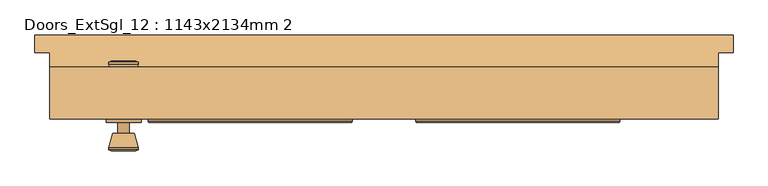
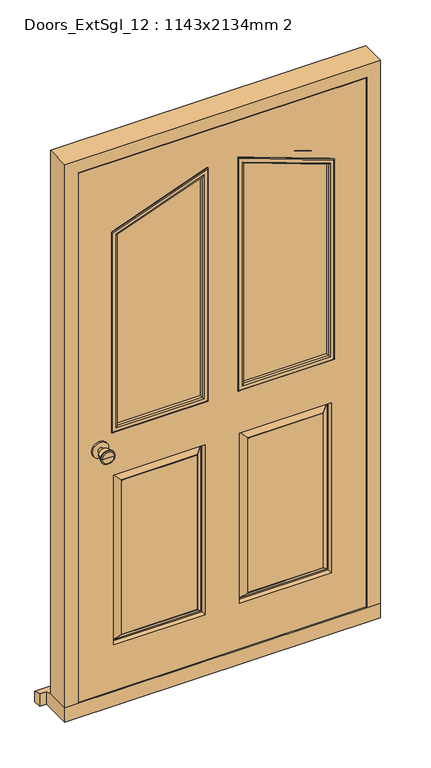
"""IFC4 building model written with IfcOpenShell, lengths in millimetres: door geometry, Doors_ExtSgl_12 : 1143x2134mm 2."""

from ifc_helpers import new_model, si_unit, point, frame, frame_2d, origin, place, context, project, spatial, polyline, circle_curve, ellipse_curve, trimmed, segment, composite_curve, outline, extrude, faceted_brep, source, transform, mapped, element, save
from ifc_brep_helpers import plane_surface, cylinder_surface, revolved_surface, advanced_brep


def doors_extsgl_12_1143x2134mm_2_6d3613a0(model_context):
    return source(origin(), model_context, "Body", "SolidModel", [
        advanced_brep(
        [(-445.0, -5.7, 1000.0), (-435.0, -5.7, 1000.0), (-455.0, -5.7, 1000.0), (-424.5241324, -54.7, 1000.0), (-445.0, -54.7, 1000.0), (-465.4758676, -54.7, 1000.0), (-420.0, -52.8721319, 1000.0), (-470.0, -52.8721319, 1000.0), (-420.0, -49.4084537, 1000.0), (-470.0, -49.4084537, 1000.0), (-426.363764, -24.7, 1000.0), (-463.636236, -24.7, 1000.0), (-435.0, -24.7, 1000.0), (-455.0, -24.7, 1000.0)],
        [
            (0, 1),
            (1, 2, circle_curve(frame((-445.0, -5.7, 1000.0), z_axis=(0.0, 1.0, 0.0), x_axis=(-1.0, 0.0, 0.0)), 10.0)),
            (2, 0),
            (2, 1, circle_curve(frame((-445.0, -5.7, 1000.0), z_axis=(0.0, 1.0, 0.0), x_axis=(-1.0, 0.0, 0.0)), 10.0)),
            (3, 4),
            (4, 5),
            (5, 3, circle_curve(frame((-445.0, -54.7, 1000.0), z_axis=(0.0, -1.0, 0.0), x_axis=(-1.0, 0.0, 0.0)), 20.4758676)),
            (3, 5, circle_curve(frame((-445.0, -54.7, 1000.0), z_axis=(0.0, -1.0, 0.0), x_axis=(-1.0, 0.0, 0.0)), 20.4758676)),
            (6, 3),
            (5, 7),
            (7, 6, circle_curve(frame((-445.0, -52.8721319, 1000.0), z_axis=(0.0, -1.0, 0.0), x_axis=(-1.0, 0.0, 0.0)), 25.0)),
            (6, 7, circle_curve(frame((-445.0, -52.8721319, 1000.0), z_axis=(0.0, -1.0, 0.0), x_axis=(-1.0, 0.0, 0.0)), 25.0)),
            (8, 6),
            (7, 9),
            (9, 8, circle_curve(frame((-445.0, -49.4084537, 1000.0), z_axis=(0.0, -1.0, 0.0), x_axis=(-1.0, 0.0, 0.0)), 25.0)),
            (8, 9, circle_curve(frame((-445.0, -49.4084537, 1000.0), z_axis=(0.0, -1.0, 0.0), x_axis=(-1.0, 0.0, 0.0)), 25.0)),
            (10, 8),
            (9, 11),
            (11, 10, circle_curve(frame((-445.0, -24.7, 1000.0), z_axis=(0.0, -1.0, 0.0), x_axis=(-1.0, 0.0, 0.0)), 18.636236)),
            (10, 11, circle_curve(frame((-445.0, -24.7, 1000.0), z_axis=(0.0, -1.0, 0.0), x_axis=(-1.0, 0.0, 0.0)), 18.636236)),
            (12, 10),
            (11, 13),
            (13, 12, circle_curve(frame((-445.0, -24.7, 1000.0), z_axis=(0.0, -1.0, 0.0), x_axis=(-1.0, 0.0, 0.0)), 10.0)),
            (12, 13, circle_curve(frame((-445.0, -24.7, 1000.0), z_axis=(0.0, -1.0, 0.0), x_axis=(-1.0, 0.0, 0.0)), 10.0)),
            (1, 12),
            (13, 2),
        ],
        [
            plane_surface(frame((-445.0, -5.7, 1000.0), z_axis=(0.0, 1.0, 0.0), x_axis=(-1.0, 0.0, 0.0))),
            plane_surface(frame((-445.0, -54.7, 1000.0), z_axis=(0.0, -1.0, 0.0), x_axis=(-1.0, 0.0, 0.0))),
            revolved_surface(polyline([(-465.4758676, -54.7, 1000.0), (-470.0, -52.8721319, 1000.0)]), (-445.0, -5.7, 1000.0), (0.0, 1.0, 0.0)),
            cylinder_surface(frame((-445.0, -5.7, 1000.0), z_axis=(0.0, 1.0, 0.0), x_axis=(-1.0, 0.0, 0.0)), 25.0),
            revolved_surface(polyline([(-470.0, -49.4084537, 1000.0), (-463.636236, -24.7, 1000.0)]), (-445.0, -5.7, 1000.0), (0.0, 1.0, 0.0)),
            plane_surface(frame((-445.0, -24.7, 1000.0), z_axis=(0.0, 1.0, 0.0), x_axis=(-1.0, 0.0, 0.0))),
            cylinder_surface(frame((-445.0, -5.7, 1000.0), z_axis=(0.0, 1.0, 0.0), x_axis=(-1.0, 0.0, 0.0)), 10.0),
        ],
        [
            (0, [[1, 2, 3]]),
            (0, [[-3, 4, -1]]),
            (1, [[5, 6, 7]]),
            (1, [[-6, -5, 8]]),
            (2, [[9, -7, 10, 11]]),
            (2, [[-10, -8, -9, 12]]),
            (3, [[13, -11, 14, 15]]),
            (3, [[-14, -12, -13, 16]]),
            (4, [[17, -15, 18, 19]]),
            (4, [[-18, -16, -17, 20]]),
            (5, [[21, -19, 22, 23]]),
            (5, [[-22, -20, -21, 24]]),
            (6, [[25, -23, 26, -2]]),
            (6, [[-26, -24, -25, -4]]),
        ],
    ),
        extrude(outline(composite_curve([segment(trimmed(circle_curve(frame_2d((1000.0, -445.0)), 30.0), [point((1000.0, -475.0))], [point((1000.0, -415.0))], False, "CARTESIAN"), True, "CONTINUOUS"), segment(trimmed(circle_curve(frame_2d((1000.0, -445.0)), 30.0), [point((1000.0, -415.0))], [point((1000.0, -475.0))], False, "CARTESIAN"), True, "CONTINUOUS")], self_intersect=False)), frame((0.0, -5.7, 0.0), z_axis=(0.0, 1.0, 0.0), x_axis=(0.0, 0.0, 1.0)), (0.0, 0.0, 1.0), 6.0),
        advanced_brep(
        [(-445.0, 50.3, 1000.0), (-455.0, 50.3, 1000.0), (-435.0, 50.3, 1000.0), (-424.5241324, 99.3, 1000.0), (-465.4758676, 99.3, 1000.0), (-445.0, 99.3, 1000.0), (-420.0, 97.4721319, 1000.0), (-470.0, 97.4721319, 1000.0), (-420.0, 94.0084537, 1000.0), (-470.0, 94.0084537, 1000.0), (-426.363764, 69.3, 1000.0), (-463.636236, 69.3, 1000.0), (-435.0, 69.3, 1000.0), (-455.0, 69.3, 1000.0)],
        [
            (0, 1),
            (1, 2, circle_curve(frame((-445.0, 50.3, 1000.0), z_axis=(0.0, -1.0, 0.0), x_axis=(-1.0, 0.0, 0.0)), 10.0)),
            (2, 0),
            (2, 1, circle_curve(frame((-445.0, 50.3, 1000.0), z_axis=(0.0, -1.0, 0.0), x_axis=(-1.0, 0.0, 0.0)), 10.0)),
            (3, 4, circle_curve(frame((-445.0, 99.3, 1000.0), z_axis=(0.0, 1.0, 0.0), x_axis=(-1.0, 0.0, 0.0)), 20.4758676)),
            (4, 5),
            (5, 3),
            (4, 3, circle_curve(frame((-445.0, 99.3, 1000.0), z_axis=(0.0, 1.0, 0.0), x_axis=(-1.0, 0.0, 0.0)), 20.4758676)),
            (6, 7, circle_curve(frame((-445.0, 97.4721319, 1000.0), z_axis=(0.0, 1.0, 0.0), x_axis=(-1.0, 0.0, 0.0)), 25.0)),
            (7, 4),
            (3, 6),
            (7, 6, circle_curve(frame((-445.0, 97.4721319, 1000.0), z_axis=(0.0, 1.0, 0.0), x_axis=(-1.0, 0.0, 0.0)), 25.0)),
            (8, 9, circle_curve(frame((-445.0, 94.0084537, 1000.0), z_axis=(0.0, 1.0, 0.0), x_axis=(-1.0, 0.0, 0.0)), 25.0)),
            (9, 7),
            (6, 8),
            (9, 8, circle_curve(frame((-445.0, 94.0084537, 1000.0), z_axis=(0.0, 1.0, 0.0), x_axis=(-1.0, 0.0, 0.0)), 25.0)),
            (10, 11, circle_curve(frame((-445.0, 69.3, 1000.0), z_axis=(0.0, 1.0, 0.0), x_axis=(-1.0, 0.0, 0.0)), 18.636236)),
            (11, 9),
            (8, 10),
            (11, 10, circle_curve(frame((-445.0, 69.3, 1000.0), z_axis=(0.0, 1.0, 0.0), x_axis=(-1.0, 0.0, 0.0)), 18.636236)),
            (12, 13, circle_curve(frame((-445.0, 69.3, 1000.0), z_axis=(0.0, 1.0, 0.0), x_axis=(-1.0, 0.0, 0.0)), 10.0)),
            (13, 11),
            (10, 12),
            (13, 12, circle_curve(frame((-445.0, 69.3, 1000.0), z_axis=(0.0, 1.0, 0.0), x_axis=(-1.0, 0.0, 0.0)), 10.0)),
            (1, 13),
            (12, 2),
        ],
        [
            plane_surface(frame((-445.0, 50.3, 1000.0), z_axis=(0.0, -1.0, 0.0), x_axis=(-1.0, 0.0, 0.0))),
            plane_surface(frame((-445.0, 99.3, 1000.0), z_axis=(0.0, 1.0, 0.0), x_axis=(-1.0, 0.0, 0.0))),
            revolved_surface(polyline([(-465.4758676, 99.3, 1000.0), (-470.0, 97.4721319, 1000.0)]), (-445.0, 50.3, 1000.0), (0.0, -1.0, 0.0)),
            cylinder_surface(frame((-445.0, 50.3, 1000.0), z_axis=(0.0, -1.0, 0.0), x_axis=(-1.0, 0.0, 0.0)), 25.0),
            revolved_surface(polyline([(-470.0, 94.0084537, 1000.0), (-463.636236, 69.3, 1000.0)]), (-445.0, 50.3, 1000.0), (0.0, -1.0, 0.0)),
            plane_surface(frame((-445.0, 69.3, 1000.0), z_axis=(0.0, -1.0, 0.0), x_axis=(-1.0, 0.0, 0.0))),
            cylinder_surface(frame((-445.0, 50.3, 1000.0), z_axis=(0.0, -1.0, 0.0), x_axis=(-1.0, 0.0, 0.0)), 10.0),
        ],
        [
            (0, [[1, 2, 3]]),
            (0, [[-3, 4, -1]]),
            (1, [[5, 6, 7]]),
            (1, [[8, -7, -6]]),
            (2, [[9, 10, -5, 11]]),
            (2, [[12, -11, -8, -10]]),
            (3, [[13, 14, -9, 15]]),
            (3, [[16, -15, -12, -14]]),
            (4, [[17, 18, -13, 19]]),
            (4, [[20, -19, -16, -18]]),
            (5, [[21, 22, -17, 23]]),
            (5, [[24, -23, -20, -22]]),
            (6, [[-2, 25, -21, 26]]),
            (6, [[-4, -26, -24, -25]]),
        ],
    ),
        extrude(outline(composite_curve([segment(trimmed(circle_curve(frame_2d((1000.0, -445.0)), 30.0), [point((1000.0, -475.0))], [point((1000.0, -415.0))], False, "CARTESIAN"), True, "CONTINUOUS"), segment(trimmed(circle_curve(frame_2d((1000.0, -445.0)), 30.0), [point((1000.0, -415.0))], [point((1000.0, -475.0))], False, "CARTESIAN"), True, "CONTINUOUS")], self_intersect=False)), frame((0.0, 44.3, 0.0), z_axis=(0.0, 1.0, 0.0), x_axis=(0.0, 0.0, 1.0)), (0.0, 0.0, 1.0), 6.0),
        faceted_brep([(501.0, 89.3, 54.5), (571.5, 89.3, 54.5), (571.5, 0.3, 54.5), (523.0, 0.3, 54.5), (523.0, 47.3, 54.5), (501.0, 47.3, 54.5), (501.0, 89.3, 2063.1), (-501.0, 89.3, 2063.1), (-501.0, 89.3, 54.5), (-571.5, 89.3, 54.5), (-571.5, 89.3, 2133.6), (571.5, 89.3, 2133.6), (571.5, 0.3, 2133.6), (-571.5, 0.3, 2133.6), (-571.5, 0.3, 54.5), (-523.0, 0.3, 54.5), (-523.0, 0.3, 2085.1), (523.0, 0.3, 2085.1), (523.0, 47.3, 2085.1), (-523.0, 47.3, 2085.1), (-523.0, 47.3, 54.5), (-501.0, 47.3, 54.5), (-501.0, 47.3, 2063.1), (501.0, 47.3, 2063.1)], [[[0, 1, 2, 3, 4, 5]], [[1, 0, 6, 7, 8, 9, 10, 11]], [[2, 1, 11, 12]], [[3, 2, 12, 13, 14, 15, 16, 17]], [[4, 3, 17, 18]], [[5, 4, 18, 19, 20, 21, 22, 23]], [[0, 5, 23, 6]], [[8, 7, 22, 21]], [[9, 8, 21, 20, 15, 14]], [[10, 9, 14, 13]], [[16, 15, 20, 19]], [[11, 10, 13, 12]], [[17, 16, 19, 18]], [[7, 6, 23, 22]]]),
        faceted_brep([(520.0, 0.3, 58.5), (520.0, 0.3, 2082.1), (-520.9250294, 0.3, 2082.1), (-520.9250294, 0.3, 58.5), (62.5, 0.3, 1058.5), (62.5, 0.3, 1932.1), (395.0, 0.3, 1811.0798971), (395.0, 0.3, 1058.5), (-395.0, 0.3, 1058.5), (-395.0, 0.3, 1811.0798971), (-62.5, 0.3, 1932.1), (-62.5, 0.3, 1058.5), (-62.5, 0.3, 883.5), (-62.5, 0.3, 233.5), (-395.0, 0.3, 233.5), (-395.0, 0.3, 883.5), (395.0, 0.3, 883.5), (395.0, 0.3, 233.5), (62.5, 0.3, 233.5), (62.5, 0.3, 883.5), (-92.5, 0.3, 263.5), (-92.5, 0.3, 853.5), (-365.0, 0.3, 853.5), (-365.0, 0.3, 263.5), (365.0, 0.3, 263.5), (365.0, 0.3, 853.5), (92.5, 0.3, 853.5), (92.5, 0.3, 263.5), (520.0, 44.3, 58.5), (-520.9250294, 44.3, 58.5), (-520.9250294, 44.3, 2082.1), (520.0, 44.3, 2082.1), (62.5, 44.3, 1058.5), (395.0, 44.3, 1058.5), (395.0, 44.3, 1811.0798971), (62.5, 44.3, 1932.1), (-395.0, 44.3, 1058.5), (-62.5, 44.3, 1058.5), (-62.5, 44.3, 1932.1), (-395.0, 44.3, 1811.0798971), (62.5, 44.3, 883.5), (62.5, 44.3, 233.5), (395.0, 44.3, 233.5), (395.0, 44.3, 883.5), (-395.0, 44.3, 883.5), (-395.0, 44.3, 233.5), (-62.5, 44.3, 233.5), (-62.5, 44.3, 883.5), (92.5, 44.3, 263.5), (92.5, 44.3, 853.5), (365.0, 44.3, 853.5), (365.0, 44.3, 263.5), (-365.0, 44.3, 263.5), (-365.0, 44.3, 853.5), (-92.5, 44.3, 853.5), (-92.5, 44.3, 263.5), (65.5, 29.3, 880.5), (65.5, 29.3, 236.5), (90.5, 43.3, 855.5), (90.5, 43.3, 261.5), (70.5, 29.3, 241.5), (70.5, 29.3, 875.5), (92.5, 43.3, 263.5), (92.5, 43.3, 853.5), (392.0, 29.3, 236.5), (367.0, 43.3, 261.5), (387.0, 29.3, 241.5), (365.0, 43.3, 263.5), (392.0, 29.3, 880.5), (367.0, 43.3, 855.5), (387.0, 29.3, 875.5), (365.0, 43.3, 853.5), (-392.0, 29.3, 880.5), (-392.0, 29.3, 236.5), (-367.0, 43.3, 855.5), (-367.0, 43.3, 261.5), (-387.0, 29.3, 241.5), (-387.0, 29.3, 875.5), (-365.0, 43.3, 263.5), (-365.0, 43.3, 853.5), (-65.5, 29.3, 236.5), (-90.5, 43.3, 261.5), (-70.5, 29.3, 241.5), (-92.5, 43.3, 263.5), (-65.5, 29.3, 880.5), (-90.5, 43.3, 855.5), (-70.5, 29.3, 875.5), (-92.5, 43.3, 853.5), (-92.5, 1.3, 263.5), (-92.5, 1.3, 853.5), (-70.5, 15.3, 241.5), (-70.5, 15.3, 875.5), (-90.5, 1.3, 855.5), (-90.5, 1.3, 261.5), (-65.5, 15.3, 880.5), (-65.5, 15.3, 236.5), (-365.0, 1.3, 853.5), (-387.0, 15.3, 875.5), (-367.0, 1.3, 855.5), (-392.0, 15.3, 880.5), (-365.0, 1.3, 263.5), (-387.0, 15.3, 241.5), (-367.0, 1.3, 261.5), (-392.0, 15.3, 236.5), (392.0, 15.3, 880.5), (392.0, 15.3, 236.5), (367.0, 1.3, 855.5), (367.0, 1.3, 261.5), (387.0, 15.3, 241.5), (387.0, 15.3, 875.5), (365.0, 1.3, 263.5), (365.0, 1.3, 853.5), (65.5, 15.3, 236.5), (90.5, 1.3, 261.5), (70.5, 15.3, 241.5), (92.5, 1.3, 263.5), (65.5, 15.3, 880.5), (90.5, 1.3, 855.5), (70.5, 15.3, 875.5), (92.5, 1.3, 853.5)], [[[0, 1, 2, 3], [4, 5, 6, 7], [8, 9, 10, 11], [12, 13, 14, 15], [16, 17, 18, 19]], [[20, 21, 22, 23]], [[24, 25, 26, 27]], [[28, 29, 30, 31], [32, 33, 34, 35], [36, 37, 38, 39], [40, 41, 42, 43], [44, 45, 46, 47]], [[48, 49, 50, 51]], [[52, 53, 54, 55]], [[1, 0, 28, 31]], [[2, 1, 31, 30]], [[3, 2, 30, 29]], [[0, 3, 29, 28]], [[5, 4, 32, 35]], [[6, 5, 35, 34]], [[7, 6, 34, 33]], [[4, 7, 33, 32]], [[9, 8, 36, 39]], [[10, 9, 39, 38]], [[11, 10, 38, 37]], [[8, 11, 37, 36]], [[56, 57, 41, 40]], [[58, 59, 60, 61]], [[48, 62, 63, 49]], [[41, 57, 64, 42]], [[60, 59, 65, 66]], [[62, 48, 51, 67]], [[42, 64, 68, 43]], [[66, 65, 69, 70]], [[67, 51, 50, 71]], [[56, 40, 43, 68]], [[57, 56, 68, 64], [61, 60, 66, 70]], [[58, 61, 70, 69]], [[59, 58, 69, 65], [63, 62, 67, 71]], [[49, 63, 71, 50]], [[72, 73, 45, 44]], [[74, 75, 76, 77]], [[52, 78, 79, 53]], [[45, 73, 80, 46]], [[76, 75, 81, 82]], [[78, 52, 55, 83]], [[46, 80, 84, 47]], [[82, 81, 85, 86]], [[83, 55, 54, 87]], [[72, 44, 47, 84]], [[73, 72, 84, 80], [77, 76, 82, 86]], [[74, 77, 86, 85]], [[75, 74, 85, 81], [79, 78, 83, 87]], [[53, 79, 87, 54]], [[88, 89, 21, 20]], [[90, 91, 92, 93]], [[12, 94, 95, 13]], [[21, 89, 96, 22]], [[92, 91, 97, 98]], [[94, 12, 15, 99]], [[22, 96, 100, 23]], [[98, 97, 101, 102]], [[99, 15, 14, 103]], [[88, 20, 23, 100]], [[93, 92, 98, 102], [89, 88, 100, 96]], [[90, 93, 102, 101]], [[95, 94, 99, 103], [91, 90, 101, 97]], [[13, 95, 103, 14]], [[104, 105, 17, 16]], [[106, 107, 108, 109]], [[24, 110, 111, 25]], [[17, 105, 112, 18]], [[108, 107, 113, 114]], [[110, 24, 27, 115]], [[18, 112, 116, 19]], [[114, 113, 117, 118]], [[115, 27, 26, 119]], [[104, 16, 19, 116]], [[105, 104, 116, 112], [109, 108, 114, 118]], [[106, 109, 118, 117]], [[107, 106, 117, 113], [111, 110, 115, 119]], [[25, 111, 119, 26]]]),
        faceted_brep([(596.5, 144.3, 0.0), (596.5, 144.3, 38.5947221), (596.5, 114.3, 47.2703282), (596.5, 114.3, 0.0), (-596.5, 144.3, 38.5947221), (-596.5, 144.3, 0.0), (-596.5, 114.3, 0.0), (-596.5, 114.3, 47.2703282), (571.5, 114.3, 0.0), (571.5, 0.3, 0.0), (-571.5, 0.3, 0.0), (-571.5, 114.3, 0.0), (-571.5, 114.3, 47.2703282), (-571.5, 89.3, 54.5), (571.5, 89.3, 54.5), (571.5, 114.3, 47.2703282), (-571.5, 0.3, 54.5), (571.5, 0.3, 54.5)], [[[0, 1, 2, 3]], [[4, 5, 6, 7]], [[5, 0, 3, 8, 9, 10, 11, 6]], [[1, 0, 5, 4]], [[1, 4, 7, 12, 13, 14, 15, 2]], [[13, 16, 17, 14]], [[16, 10, 9, 17]], [[12, 11, 10, 16, 13]], [[11, 12, 7, 6]], [[8, 15, 14, 17, 9]], [[15, 8, 3, 2]]]),
        extrude(outline(polyline([(1058.5, 395.0), (1811.0798971, 395.0), (1932.1, 62.5), (1058.5, 62.5), (1058.5, 395.0)])), frame((0.0, 10.3, 0.0), z_axis=(0.0, 1.0, 0.0), x_axis=(0.0, 0.0, 1.0)), (0.0, 0.0, 1.0), 24.0),
        extrude(outline(polyline([(1058.5, -62.5), (1932.1, -62.5), (1811.0798971, -395.0), (1058.5, -395.0), (1058.5, -62.5)])), frame((0.0, 10.3, 0.0), z_axis=(0.0, 1.0, 0.0), x_axis=(0.0, 0.0, 1.0)), (0.0, 0.0, 1.0), 24.0),
        advanced_brep(
        [(403.0, 48.3, 1816.6815574), (403.0, 44.3, 1816.6815574), (403.0, 44.3, 1050.5), (403.0, 48.3, 1050.5), (401.0, 50.3, 1815.2811423), (401.0, 50.3, 1052.5), (383.0, 45.3, 1802.6774066), (388.0, 50.3, 1806.1784443), (388.0, 50.3, 1065.5), (383.0, 45.3, 1070.5), (383.0, 34.3, 1802.6774066), (383.0, 34.3, 1070.5), (395.0, 44.3, 1811.0798971), (395.0, 34.3, 1811.0798971), (395.0, 34.3, 1058.5), (395.0, 44.3, 1058.5), (54.5, 44.3, 1050.5), (54.5, 48.3, 1050.5), (56.5, 50.3, 1052.5), (69.5, 50.3, 1065.5), (74.5, 45.3, 1070.5), (74.5, 34.3, 1070.5), (62.5, 34.3, 1058.5), (62.5, 44.3, 1058.5), (54.5, 44.3, 1943.5251841), (54.5, 48.3, 1943.5251841), (56.5, 50.3, 1940.668888), (69.5, 50.3, 1922.102964), (74.5, 45.3, 1914.9622239), (74.5, 34.3, 1914.9622239), (62.5, 34.3, 1932.1), (62.5, 44.3, 1932.1)],
        [
            (0, 1),
            (1, 2),
            (2, 3),
            (3, 0),
            (4, 0, ellipse_curve(frame((401.0, 48.3, 1815.2811423), z_axis=(0.5735764363510462, 0.0, -0.8191520442889917), x_axis=(0.8191520442889916, 0.0, 0.5735764363510463)), 2.4415492, 2.0)),
            (3, 5, ellipse_curve(frame((401.0, 48.3, 1052.5), z_axis=(0.7071067811865475, 0.0, 0.7071067811865475), x_axis=(-0.7071067811865474, 0.0, 0.7071067811865476)), 2.8284271, 2.0)),
            (5, 4),
            (6, 7, ellipse_curve(frame((388.0, 45.3, 1806.1784443), z_axis=(0.5735764363510462, 0.0, -0.8191520442889917), x_axis=(0.8191520442889916, 0.0, 0.5735764363510463)), 6.1038729, 5.0)),
            (7, 8),
            (8, 9, ellipse_curve(frame((388.0, 45.3, 1065.5), z_axis=(0.7071067811865475, 0.0, 0.7071067811865475), x_axis=(-0.7071067811865474, 0.0, 0.7071067811865476)), 7.0710678, 5.0)),
            (9, 6),
            (10, 6),
            (9, 11),
            (11, 10),
            (12, 13),
            (13, 14),
            (14, 15),
            (15, 12),
            (2, 16),
            (16, 17),
            (17, 3),
            (17, 18, ellipse_curve(frame((56.5, 48.3, 1052.5), z_axis=(0.7071067811865475, 0.0, -0.7071067811865475), x_axis=(0.7071067811865476, 0.0, 0.7071067811865474)), 2.8284271, 2.0)),
            (18, 5),
            (8, 19),
            (19, 20, ellipse_curve(frame((69.5, 45.3, 1065.5), z_axis=(0.7071067811865475, 0.0, -0.7071067811865475), x_axis=(0.7071067811865476, 0.0, 0.7071067811865474)), 7.0710678, 5.0)),
            (20, 9),
            (20, 21),
            (21, 11),
            (14, 22),
            (22, 23),
            (23, 15),
            (16, 24),
            (24, 25),
            (25, 17),
            (25, 26, ellipse_curve(frame((56.5, 48.3, 1940.668888), z_axis=(-0.8191520442889917, 0.0, -0.573576436351046), x_axis=(0.5735764363510459, 0.0, -0.8191520442889919)), 3.4868936, 2.0)),
            (26, 18),
            (19, 27),
            (27, 28, ellipse_curve(frame((69.5, 45.3, 1922.102964), z_axis=(-0.8191520442889917, 0.0, -0.573576436351046), x_axis=(0.5735764363510459, 0.0, -0.8191520442889919)), 8.717234, 5.0)),
            (28, 20),
            (28, 29),
            (29, 21),
            (22, 30),
            (30, 31),
            (31, 23),
            (24, 1),
            (0, 25),
            (4, 26),
            (7, 27),
            (6, 28),
            (10, 29),
            (13, 30),
            (12, 31),
        ],
        [
            plane_surface(frame((403.0, 44.3, 1816.6815574), z_axis=(1.0, 0.0, 0.0), x_axis=(0.0, 0.0, -1.0))),
            cylinder_surface(frame((401.0, 48.3, 1811.0798971), z_axis=(0.0, 0.0, 1.0), x_axis=(1.0, 0.0, 0.0)), 2.0),
            cylinder_surface(frame((388.0, 45.3, 1811.0798971), z_axis=(0.0, 0.0, 1.0), x_axis=(1.0, 0.0, 0.0)), 5.0),
            plane_surface(frame((383.0, 45.3, 1802.6774066), z_axis=(-1.0, 0.0, 0.0), x_axis=(0.0, 0.0, -1.0))),
            plane_surface(frame((395.0, 34.3, 1811.0798971), z_axis=(1.0, 0.0, 0.0), x_axis=(0.0, 0.0, -1.0))),
            plane_surface(frame((403.0, 44.3, 1050.5), z_axis=(0.0, 0.0, -1.0), x_axis=(-1.0, 0.0, 0.0))),
            cylinder_surface(frame((395.0, 48.3, 1052.5), z_axis=(1.0, 0.0, 0.0), x_axis=(0.0, 0.0, -1.0)), 2.0),
            cylinder_surface(frame((395.0, 45.3, 1065.5), z_axis=(1.0, 0.0, 0.0), x_axis=(0.0, 0.0, -1.0)), 5.0),
            plane_surface(frame((383.0, 45.3, 1070.5), z_axis=(0.0, 0.0, 1.0), x_axis=(-1.0, 0.0, 0.0))),
            plane_surface(frame((395.0, 34.3, 1058.5), z_axis=(0.0, 0.0, -1.0), x_axis=(-1.0, 0.0, 0.0))),
            plane_surface(frame((54.5, 44.3, 1050.5), z_axis=(-1.0, 0.0, 0.0), x_axis=(0.0, 0.0, 1.0))),
            cylinder_surface(frame((56.5, 48.3, 1058.5), z_axis=(0.0, 0.0, -1.0), x_axis=(-1.0, 0.0, 0.0)), 2.0),
            cylinder_surface(frame((69.5, 45.3, 1058.5), z_axis=(0.0, 0.0, -1.0), x_axis=(-1.0, 0.0, 0.0)), 5.0),
            plane_surface(frame((74.5, 45.3, 1070.5), z_axis=(1.0, 0.0, 0.0), x_axis=(0.0, 0.0, 1.0))),
            plane_surface(frame((62.5, 34.3, 1058.5), z_axis=(-1.0, 0.0, 0.0), x_axis=(0.0, 0.0, 1.0))),
            plane_surface(frame((54.5, 44.3, 1943.5251841), z_axis=(0.34202014332566855, 0.0, 0.9396926207859085), x_axis=(0.9396926207859085, 0.0, -0.34202014332566855))),
            cylinder_surface(frame((64.5521209, 48.3, 1937.7381557), z_axis=(-0.9396926207859084, 0.0, 0.3420201433256686), x_axis=(0.3420201433256686, 0.0, 0.9396926207859084)), 2.0),
            plane_surface(frame((56.5, 50.3, 1940.668888), z_axis=(0.0, 1.0, 0.0), x_axis=(0.9396926207859083, 0.0, -0.342020143325669))),
            cylinder_surface(frame((60.105859, 45.3, 1925.5221517), z_axis=(-0.9396926207859084, 0.0, 0.3420201433256686), x_axis=(0.3420201433256686, 0.0, 0.9396926207859084)), 5.0),
            plane_surface(frame((74.5, 45.3, 1914.9622239), z_axis=(-0.34202014332566855, 0.0, -0.9396926207859085), x_axis=(0.9396926207859085, 0.0, -0.34202014332566855))),
            plane_surface(frame((74.5, 34.3, 1914.9622239), z_axis=(0.0, -1.0, 0.0), x_axis=(0.9396926207859084, 0.0, -0.34202014332566866))),
            plane_surface(frame((62.5, 34.3, 1932.1), z_axis=(0.3420201433256685, 0.0, 0.9396926207859085), x_axis=(0.9396926207859085, 0.0, -0.3420201433256685))),
            plane_surface(frame((62.5, 44.3, 1932.1), z_axis=(0.0, -1.0, 0.0), x_axis=(0.9396926207859085, 0.0, -0.3420201433256685))),
        ],
        [
            (0, [[1, 2, 3, 4]]),
            (1, [[5, -4, 6, 7]]),
            (2, [[8, 9, 10, 11]]),
            (3, [[12, -11, 13, 14]]),
            (4, [[15, 16, 17, 18]]),
            (5, [[-3, 19, 20, 21]]),
            (6, [[-6, -21, 22, 23]]),
            (7, [[-10, 24, 25, 26]]),
            (8, [[-13, -26, 27, 28]]),
            (9, [[-17, 29, 30, 31]]),
            (10, [[-20, 32, 33, 34]]),
            (11, [[-22, -34, 35, 36]]),
            (12, [[-25, 37, 38, 39]]),
            (13, [[-27, -39, 40, 41]]),
            (14, [[-30, 42, 43, 44]]),
            (15, [[-33, 45, -1, 46]]),
            (16, [[-35, -46, -5, 47]]),
            (17, [[-23, -36, -47, -7], [48, -37, -24, -9]]),
            (18, [[-38, -48, -8, 49]]),
            (19, [[-40, -49, -12, 50]]),
            (20, [[51, -42, -29, -16], [-28, -41, -50, -14]]),
            (21, [[-43, -51, -15, 52]]),
            (22, [[-45, -32, -19, -2], [-31, -44, -52, -18]]),
        ],
    ),
        advanced_brep(
        [(-54.5, 48.3, 1050.5), (-54.5, 44.3, 1050.5), (-403.0, 44.3, 1050.5), (-403.0, 48.3, 1050.5), (-56.5, 50.3, 1052.5), (-401.0, 50.3, 1052.5), (-74.5, 45.3, 1070.5), (-69.5, 50.3, 1065.5), (-388.0, 50.3, 1065.5), (-383.0, 45.3, 1070.5), (-74.5, 34.3, 1070.5), (-383.0, 34.3, 1070.5), (-62.5, 44.3, 1058.5), (-62.5, 34.3, 1058.5), (-395.0, 34.3, 1058.5), (-395.0, 44.3, 1058.5), (-403.0, 44.3, 1816.6815574), (-403.0, 48.3, 1816.6815574), (-401.0, 50.3, 1815.2811423), (-388.0, 50.3, 1806.1784443), (-383.0, 45.3, 1802.6774066), (-383.0, 34.3, 1802.6774066), (-395.0, 34.3, 1811.0798971), (-395.0, 44.3, 1811.0798971), (-54.5, 44.3, 1943.5251841), (-54.5, 48.3, 1943.5251841), (-56.5, 50.3, 1940.668888), (-69.5, 50.3, 1922.102964), (-74.5, 45.3, 1914.9622239), (-74.5, 34.3, 1914.9622239), (-62.5, 34.3, 1932.1), (-62.5, 44.3, 1932.1)],
        [
            (0, 1),
            (1, 2),
            (2, 3),
            (3, 0),
            (4, 0, ellipse_curve(frame((-56.5, 48.3, 1052.5), z_axis=(-0.7071067811865476, 0.0, -0.7071067811865474), x_axis=(0.7071067811865476, 0.0, -0.7071067811865475)), 2.8284271, 2.0)),
            (3, 5, ellipse_curve(frame((-401.0, 48.3, 1052.5), z_axis=(0.7071067811865474, 0.0, -0.7071067811865476), x_axis=(0.7071067811865478, 0.0, 0.7071067811865474)), 2.8284271, 2.0)),
            (5, 4),
            (6, 7, ellipse_curve(frame((-69.5, 45.3, 1065.5), z_axis=(-0.7071067811865476, 0.0, -0.7071067811865474), x_axis=(0.7071067811865476, 0.0, -0.7071067811865475)), 7.0710678, 5.0)),
            (7, 8),
            (8, 9, ellipse_curve(frame((-388.0, 45.3, 1065.5), z_axis=(0.7071067811865474, 0.0, -0.7071067811865476), x_axis=(0.7071067811865478, 0.0, 0.7071067811865474)), 7.0710678, 5.0)),
            (9, 6),
            (10, 6),
            (9, 11),
            (11, 10),
            (12, 13),
            (13, 14),
            (14, 15),
            (15, 12),
            (2, 16),
            (16, 17),
            (17, 3),
            (17, 18, ellipse_curve(frame((-401.0, 48.3, 1815.2811423), z_axis=(-0.5735764363510212, 0.0, -0.8191520442890091), x_axis=(0.8191520442890092, 0.0, -0.5735764363510214)), 2.4415492, 2.0)),
            (18, 5),
            (8, 19),
            (19, 20, ellipse_curve(frame((-388.0, 45.3, 1806.1784443), z_axis=(-0.5735764363510212, 0.0, -0.8191520442890091), x_axis=(0.8191520442890092, 0.0, -0.5735764363510214)), 6.1038729, 5.0)),
            (20, 9),
            (20, 21),
            (21, 11),
            (14, 22),
            (22, 23),
            (23, 15),
            (16, 24),
            (24, 25),
            (25, 17),
            (25, 26, ellipse_curve(frame((-56.5, 48.3, 1940.668888), z_axis=(-0.8191520442890093, 0.0, 0.5735764363510213), x_axis=(-0.573576436351021, 0.0, -0.8191520442890092)), 3.4868936, 2.0)),
            (26, 18),
            (19, 27),
            (27, 28, ellipse_curve(frame((-69.5, 45.3, 1922.102964), z_axis=(-0.8191520442890093, 0.0, 0.5735764363510213), x_axis=(-0.573576436351021, 0.0, -0.8191520442890092)), 8.717234, 5.0)),
            (28, 20),
            (28, 29),
            (29, 21),
            (22, 30),
            (30, 31),
            (31, 23),
            (24, 1),
            (0, 25),
            (4, 26),
            (7, 27),
            (6, 28),
            (10, 29),
            (13, 30),
            (12, 31),
        ],
        [
            plane_surface(frame((-54.5, 44.3, 1050.5), z_axis=(0.0, 0.0, -1.0), x_axis=(-1.0, 0.0, 0.0))),
            cylinder_surface(frame((-62.5, 48.3, 1052.5), z_axis=(1.0, 0.0, 0.0), x_axis=(0.0, 0.0, -1.0)), 2.0),
            cylinder_surface(frame((-62.5, 45.3, 1065.5), z_axis=(1.0, 0.0, 0.0), x_axis=(0.0, 0.0, -1.0)), 5.0),
            plane_surface(frame((-74.5, 45.3, 1070.5), z_axis=(0.0, 0.0, 1.0), x_axis=(-1.0, 0.0, 0.0))),
            plane_surface(frame((-62.5, 34.3, 1058.5), z_axis=(0.0, 0.0, -1.0), x_axis=(-1.0, 0.0, 0.0))),
            plane_surface(frame((-403.0, 44.3, 1050.5), z_axis=(-1.0, 0.0, 0.0), x_axis=(0.0, 0.0, 1.0))),
            cylinder_surface(frame((-401.0, 48.3, 1058.5), z_axis=(0.0, 0.0, -1.0), x_axis=(-1.0, 0.0, 0.0)), 2.0),
            cylinder_surface(frame((-388.0, 45.3, 1058.5), z_axis=(0.0, 0.0, -1.0), x_axis=(-1.0, 0.0, 0.0)), 5.0),
            plane_surface(frame((-383.0, 45.3, 1070.5), z_axis=(1.0, 0.0, 0.0), x_axis=(0.0, 0.0, 1.0))),
            plane_surface(frame((-395.0, 34.3, 1058.5), z_axis=(-1.0, 0.0, 0.0), x_axis=(0.0, 0.0, 1.0))),
            plane_surface(frame((-403.0, 44.3, 1816.6815574), z_axis=(-0.3420201433257257, 0.0, 0.9396926207858877), x_axis=(0.9396926207858877, 0.0, 0.3420201433257257))),
            cylinder_surface(frame((-397.0521209, 48.3, 1816.7180528), z_axis=(-0.9396926207858877, 0.0, -0.3420201433257259), x_axis=(-0.3420201433257259, 0.0, 0.9396926207858877)), 2.0),
            cylinder_surface(frame((-392.605859, 45.3, 1804.5020488), z_axis=(-0.9396926207858877, 0.0, -0.3420201433257259), x_axis=(-0.3420201433257259, 0.0, 0.9396926207858877)), 5.0),
            plane_surface(frame((-383.0, 45.3, 1802.6774066), z_axis=(0.34202014332572545, 0.0, -0.9396926207858878), x_axis=(0.9396926207858878, 0.0, 0.34202014332572545))),
            plane_surface(frame((-395.0, 34.3, 1811.0798971), z_axis=(-0.342020143325726, 0.0, 0.9396926207858876), x_axis=(0.9396926207858876, 0.0, 0.342020143325726))),
            plane_surface(frame((-54.5, 44.3, 1943.5251841), z_axis=(1.0, 0.0, 0.0), x_axis=(0.0, 0.0, -1.0))),
            cylinder_surface(frame((-56.5, 48.3, 1932.1), z_axis=(0.0, 0.0, 1.0), x_axis=(1.0, 0.0, 0.0)), 2.0),
            plane_surface(frame((-56.5, 50.3, 1940.668888), z_axis=(0.0, 1.0, 0.0), x_axis=(0.0, 0.0, -1.0))),
            cylinder_surface(frame((-69.5, 45.3, 1932.1), z_axis=(0.0, 0.0, 1.0), x_axis=(1.0, 0.0, 0.0)), 5.0),
            plane_surface(frame((-74.5, 45.3, 1914.9622239), z_axis=(-1.0, 0.0, 0.0), x_axis=(0.0, 0.0, -1.0))),
            plane_surface(frame((-74.5, 34.3, 1914.9622239), z_axis=(0.0, -1.0, 0.0), x_axis=(0.0, 0.0, -1.0))),
            plane_surface(frame((-62.5, 34.3, 1932.1), z_axis=(1.0, 0.0, 0.0), x_axis=(0.0, 0.0, -1.0))),
            plane_surface(frame((-62.5, 44.3, 1932.1), z_axis=(0.0, -1.0, 0.0), x_axis=(0.0, 0.0, -1.0))),
        ],
        [
            (0, [[1, 2, 3, 4]]),
            (1, [[5, -4, 6, 7]]),
            (2, [[8, 9, 10, 11]]),
            (3, [[12, -11, 13, 14]]),
            (4, [[15, 16, 17, 18]]),
            (5, [[-3, 19, 20, 21]]),
            (6, [[-6, -21, 22, 23]]),
            (7, [[-10, 24, 25, 26]]),
            (8, [[-13, -26, 27, 28]]),
            (9, [[-17, 29, 30, 31]]),
            (10, [[-20, 32, 33, 34]]),
            (11, [[-22, -34, 35, 36]]),
            (12, [[-25, 37, 38, 39]]),
            (13, [[-27, -39, 40, 41]]),
            (14, [[-30, 42, 43, 44]]),
            (15, [[-33, 45, -1, 46]]),
            (16, [[-35, -46, -5, 47]]),
            (17, [[-23, -36, -47, -7], [48, -37, -24, -9]]),
            (18, [[-38, -48, -8, 49]]),
            (19, [[-40, -49, -12, 50]]),
            (20, [[51, -42, -29, -16], [-28, -41, -50, -14]]),
            (21, [[-43, -51, -15, 52]]),
            (22, [[-45, -32, -19, -2], [-31, -44, -52, -18]]),
        ],
    ),
        advanced_brep(
        [(-395.0, 10.3, 1811.0798971), (-395.0, 0.3, 1811.0798971), (-62.5, 0.3, 1932.1), (-62.5, 10.3, 1932.1), (-383.0, -0.7, 1802.6774066), (-383.0, 10.3, 1802.6774066), (-74.5, 10.3, 1914.9622239), (-74.5, -0.7, 1914.9622239), (-388.0, -5.7, 1806.1784443), (-69.5, -5.7, 1922.102964), (-403.0, -3.7, 1816.6815574), (-401.0, -5.7, 1815.2811423), (-56.5, -5.7, 1940.668888), (-54.5, -3.7, 1943.5251841), (-403.0, 0.3, 1816.6815574), (-54.5, 0.3, 1943.5251841), (-62.5, 0.3, 1058.5), (-62.5, 10.3, 1058.5), (-74.5, 10.3, 1070.5), (-74.5, -0.7, 1070.5), (-69.5, -5.7, 1065.5), (-56.5, -5.7, 1052.5), (-54.5, -3.7, 1050.5), (-54.5, 0.3, 1050.5), (-395.0, 0.3, 1058.5), (-395.0, 10.3, 1058.5), (-383.0, 10.3, 1070.5), (-383.0, -0.7, 1070.5), (-388.0, -5.7, 1065.5), (-401.0, -5.7, 1052.5), (-403.0, -3.7, 1050.5), (-403.0, 0.3, 1050.5)],
        [
            (0, 1),
            (1, 2),
            (2, 3),
            (3, 0),
            (4, 5),
            (5, 6),
            (6, 7),
            (7, 4),
            (8, 4, ellipse_curve(frame((-388.0, -0.7, 1806.1784443), z_axis=(0.5735764363510213, 0.0, 0.8191520442890091), x_axis=(-0.8191520442890091, 0.0, 0.5735764363510212)), 6.1038729, 5.0)),
            (7, 9, ellipse_curve(frame((-69.5, -0.7, 1922.102964), z_axis=(-0.819152044289009, 0.0, 0.5735764363510213), x_axis=(-0.5735764363510215, 0.0, -0.819152044289009)), 8.717234, 5.0)),
            (9, 8),
            (10, 11, ellipse_curve(frame((-401.0, -3.7, 1815.2811423), z_axis=(0.5735764363510213, 0.0, 0.8191520442890091), x_axis=(-0.8191520442890091, 0.0, 0.5735764363510212)), 2.4415492, 2.0)),
            (11, 12),
            (12, 13, ellipse_curve(frame((-56.5, -3.7, 1940.668888), z_axis=(-0.819152044289009, 0.0, 0.5735764363510213), x_axis=(-0.5735764363510215, 0.0, -0.819152044289009)), 3.4868936, 2.0)),
            (13, 10),
            (14, 10),
            (13, 15),
            (15, 14),
            (2, 16),
            (16, 17),
            (17, 3),
            (6, 18),
            (18, 19),
            (19, 7),
            (19, 20, ellipse_curve(frame((-69.5, -0.7, 1065.5), z_axis=(0.7071067811865474, 0.0, 0.7071067811865476), x_axis=(-0.7071067811865475, 0.0, 0.7071067811865475)), 7.0710678, 5.0)),
            (20, 9),
            (12, 21),
            (21, 22, ellipse_curve(frame((-56.5, -3.7, 1052.5), z_axis=(0.7071067811865474, 0.0, 0.7071067811865476), x_axis=(-0.7071067811865475, 0.0, 0.7071067811865475)), 2.8284271, 2.0)),
            (22, 13),
            (22, 23),
            (23, 15),
            (16, 24),
            (24, 25),
            (25, 17),
            (18, 26),
            (26, 27),
            (27, 19),
            (27, 28, ellipse_curve(frame((-388.0, -0.7, 1065.5), z_axis=(0.7071067811865476, 0.0, -0.7071067811865474), x_axis=(0.7071067811865475, 0.0, 0.7071067811865475)), 7.0710678, 5.0)),
            (28, 20),
            (21, 29),
            (29, 30, ellipse_curve(frame((-401.0, -3.7, 1052.5), z_axis=(0.7071067811865476, 0.0, -0.7071067811865474), x_axis=(0.7071067811865475, 0.0, 0.7071067811865475)), 2.8284271, 2.0)),
            (30, 22),
            (30, 31),
            (31, 23),
            (31, 14),
            (1, 24),
            (0, 25),
            (5, 26),
            (4, 27),
            (8, 28),
            (11, 29),
            (10, 30),
        ],
        [
            plane_surface(frame((-395.0, 0.3, 1811.0798971), z_axis=(-0.3420201433257253, 0.0, 0.9396926207858879), x_axis=(0.9396926207858879, 0.0, 0.3420201433257253))),
            plane_surface(frame((-383.0, 10.3, 1802.6774066), z_axis=(0.34202014332572483, 0.0, -0.939692620785888), x_axis=(0.939692620785888, 0.0, 0.34202014332572483))),
            cylinder_surface(frame((-392.605859, -0.7, 1804.5020488), z_axis=(-0.9396926207858879, 0.0, -0.3420201433257255), x_axis=(-0.3420201433257255, 0.0, 0.9396926207858879)), 5.0),
            cylinder_surface(frame((-397.0521209, -3.7, 1816.7180528), z_axis=(-0.9396926207858879, 0.0, -0.3420201433257255), x_axis=(-0.3420201433257255, 0.0, 0.9396926207858879)), 2.0),
            plane_surface(frame((-403.0, -3.7, 1816.6815574), z_axis=(-0.34202014332572556, 0.0, 0.9396926207858878), x_axis=(0.9396926207858878, 0.0, 0.34202014332572556))),
            plane_surface(frame((-62.5, 0.3, 1932.1), z_axis=(1.0, 0.0, 0.0), x_axis=(0.0, 0.0, -1.0))),
            plane_surface(frame((-74.5, 10.3, 1914.9622239), z_axis=(-1.0, 0.0, 0.0), x_axis=(0.0, 0.0, -1.0))),
            cylinder_surface(frame((-69.5, -0.7, 1932.1), z_axis=(0.0, 0.0, 1.0), x_axis=(1.0, 0.0, 0.0)), 5.0),
            cylinder_surface(frame((-56.5, -3.7, 1932.1), z_axis=(0.0, 0.0, 1.0), x_axis=(1.0, 0.0, 0.0)), 2.0),
            plane_surface(frame((-54.5, -3.7, 1943.5251841), z_axis=(1.0, 0.0, 0.0), x_axis=(0.0, 0.0, -1.0))),
            plane_surface(frame((-62.5, 0.3, 1058.5), z_axis=(0.0, 0.0, -1.0), x_axis=(-1.0, 0.0, 0.0))),
            plane_surface(frame((-74.5, 10.3, 1070.5), z_axis=(0.0, 0.0, 1.0), x_axis=(-1.0, 0.0, 0.0))),
            cylinder_surface(frame((-62.5, -0.7, 1065.5), z_axis=(1.0, 0.0, 0.0), x_axis=(0.0, 0.0, -1.0)), 5.0),
            cylinder_surface(frame((-62.5, -3.7, 1052.5), z_axis=(1.0, 0.0, 0.0), x_axis=(0.0, 0.0, -1.0)), 2.0),
            plane_surface(frame((-54.5, -3.7, 1050.5), z_axis=(0.0, 0.0, -1.0), x_axis=(-1.0, 0.0, 0.0))),
            plane_surface(frame((-403.0, 0.3, 1050.5), z_axis=(0.0, 1.0, 0.0), x_axis=(0.0, 0.0, 1.0))),
            plane_surface(frame((-395.0, 0.3, 1058.5), z_axis=(-1.0, 0.0, 0.0), x_axis=(0.0, 0.0, 1.0))),
            plane_surface(frame((-395.0, 10.3, 1058.5), z_axis=(0.0, 1.0, 0.0), x_axis=(0.0, 0.0, 1.0))),
            plane_surface(frame((-383.0, 10.3, 1070.5), z_axis=(1.0, 0.0, 0.0), x_axis=(0.0, 0.0, 1.0))),
            cylinder_surface(frame((-388.0, -0.7, 1058.5), z_axis=(0.0, 0.0, -1.0), x_axis=(-1.0, 0.0, 0.0)), 5.0),
            plane_surface(frame((-388.0, -5.7, 1065.5), z_axis=(0.0, -1.0, 0.0), x_axis=(0.0, 0.0, 1.0))),
            cylinder_surface(frame((-401.0, -3.7, 1058.5), z_axis=(0.0, 0.0, -1.0), x_axis=(-1.0, 0.0, 0.0)), 2.0),
            plane_surface(frame((-403.0, -3.7, 1050.5), z_axis=(-1.0, 0.0, 0.0), x_axis=(0.0, 0.0, 1.0))),
        ],
        [
            (0, [[1, 2, 3, 4]]),
            (1, [[5, 6, 7, 8]]),
            (2, [[9, -8, 10, 11]]),
            (3, [[12, 13, 14, 15]]),
            (4, [[16, -15, 17, 18]]),
            (5, [[-3, 19, 20, 21]]),
            (6, [[-7, 22, 23, 24]]),
            (7, [[-10, -24, 25, 26]]),
            (8, [[-14, 27, 28, 29]]),
            (9, [[-17, -29, 30, 31]]),
            (10, [[-20, 32, 33, 34]]),
            (11, [[-23, 35, 36, 37]]),
            (12, [[-25, -37, 38, 39]]),
            (13, [[-28, 40, 41, 42]]),
            (14, [[-30, -42, 43, 44]]),
            (15, [[-31, -44, 45, -18], [46, -32, -19, -2]]),
            (16, [[-33, -46, -1, 47]]),
            (17, [[-21, -34, -47, -4], [48, -35, -22, -6]]),
            (18, [[-36, -48, -5, 49]]),
            (19, [[-38, -49, -9, 50]]),
            (20, [[51, -40, -27, -13], [-26, -39, -50, -11]]),
            (21, [[-41, -51, -12, 52]]),
            (22, [[-43, -52, -16, -45]]),
        ],
    ),
        advanced_brep(
        [(62.5, 10.3, 1932.1), (62.5, 0.3, 1932.1), (395.0, 0.3, 1811.0798971), (395.0, 10.3, 1811.0798971), (74.5, -0.7, 1914.9622239), (74.5, 10.3, 1914.9622239), (383.0, 10.3, 1802.6774066), (383.0, -0.7, 1802.6774066), (69.5, -5.7, 1922.102964), (388.0, -5.7, 1806.1784443), (54.5, -3.7, 1943.5251841), (56.5, -5.7, 1940.668888), (401.0, -5.7, 1815.2811423), (403.0, -3.7, 1816.6815574), (54.5, 0.3, 1943.5251841), (403.0, 0.3, 1816.6815574), (395.0, 0.3, 1058.5), (395.0, 10.3, 1058.5), (383.0, 10.3, 1070.5), (383.0, -0.7, 1070.5), (388.0, -5.7, 1065.5), (401.0, -5.7, 1052.5), (403.0, -3.7, 1050.5), (403.0, 0.3, 1050.5), (62.5, 0.3, 1058.5), (62.5, 10.3, 1058.5), (74.5, 10.3, 1070.5), (74.5, -0.7, 1070.5), (69.5, -5.7, 1065.5), (56.5, -5.7, 1052.5), (54.5, -3.7, 1050.5), (54.5, 0.3, 1050.5)],
        [
            (0, 1),
            (1, 2),
            (2, 3),
            (3, 0),
            (4, 5),
            (5, 6),
            (6, 7),
            (7, 4),
            (8, 4, ellipse_curve(frame((69.5, -0.7, 1922.102964), z_axis=(0.8191520442889915, 0.0, 0.5735764363510464), x_axis=(-0.5735764363510465, 0.0, 0.8191520442889915)), 8.717234, 5.0)),
            (7, 9, ellipse_curve(frame((388.0, -0.7, 1806.1784443), z_axis=(-0.5735764363510464, 0.0, 0.8191520442889916), x_axis=(-0.8191520442889916, 0.0, -0.5735764363510463)), 6.1038729, 5.0)),
            (9, 8),
            (10, 11, ellipse_curve(frame((56.5, -3.7, 1940.668888), z_axis=(0.8191520442889915, 0.0, 0.5735764363510464), x_axis=(-0.5735764363510465, 0.0, 0.8191520442889915)), 3.4868936, 2.0)),
            (11, 12),
            (12, 13, ellipse_curve(frame((401.0, -3.7, 1815.2811423), z_axis=(-0.5735764363510464, 0.0, 0.8191520442889916), x_axis=(-0.8191520442889916, 0.0, -0.5735764363510463)), 2.4415492, 2.0)),
            (13, 10),
            (14, 10),
            (13, 15),
            (15, 14),
            (2, 16),
            (16, 17),
            (17, 3),
            (6, 18),
            (18, 19),
            (19, 7),
            (19, 20, ellipse_curve(frame((388.0, -0.7, 1065.5), z_axis=(0.7071067811865474, 0.0, 0.7071067811865477), x_axis=(-0.7071067811865478, 0.0, 0.7071067811865474)), 7.0710678, 5.0)),
            (20, 9),
            (12, 21),
            (21, 22, ellipse_curve(frame((401.0, -3.7, 1052.5), z_axis=(0.7071067811865474, 0.0, 0.7071067811865477), x_axis=(-0.7071067811865478, 0.0, 0.7071067811865474)), 2.8284271, 2.0)),
            (22, 13),
            (22, 23),
            (23, 15),
            (16, 24),
            (24, 25),
            (25, 17),
            (18, 26),
            (26, 27),
            (27, 19),
            (27, 28, ellipse_curve(frame((69.5, -0.7, 1065.5), z_axis=(0.7071067811865477, 0.0, -0.7071067811865474), x_axis=(0.7071067811865474, 0.0, 0.7071067811865476)), 7.0710678, 5.0)),
            (28, 20),
            (21, 29),
            (29, 30, ellipse_curve(frame((56.5, -3.7, 1052.5), z_axis=(0.7071067811865477, 0.0, -0.7071067811865474), x_axis=(0.7071067811865474, 0.0, 0.7071067811865476)), 2.8284271, 2.0)),
            (30, 22),
            (30, 31),
            (31, 23),
            (31, 14),
            (1, 24),
            (0, 25),
            (5, 26),
            (4, 27),
            (8, 28),
            (11, 29),
            (10, 30),
        ],
        [
            plane_surface(frame((62.5, 0.3, 1932.1), z_axis=(0.3420201433256682, 0.0, 0.9396926207859086), x_axis=(0.9396926207859086, 0.0, -0.3420201433256682))),
            plane_surface(frame((74.5, 10.3, 1914.9622239), z_axis=(-0.3420201433256686, 0.0, -0.9396926207859085), x_axis=(0.9396926207859085, 0.0, -0.3420201433256686))),
            cylinder_surface(frame((60.105859, -0.7, 1925.5221517), z_axis=(-0.9396926207859085, 0.0, 0.3420201433256683), x_axis=(0.3420201433256683, 0.0, 0.9396926207859085)), 5.0),
            cylinder_surface(frame((64.5521209, -3.7, 1937.7381557), z_axis=(-0.9396926207859085, 0.0, 0.3420201433256683), x_axis=(0.3420201433256683, 0.0, 0.9396926207859085)), 2.0),
            plane_surface(frame((54.5, -3.7, 1943.5251841), z_axis=(0.34202014332566866, 0.0, 0.9396926207859084), x_axis=(0.9396926207859084, 0.0, -0.34202014332566866))),
            plane_surface(frame((395.0, 0.3, 1811.0798971), z_axis=(1.0, 0.0, 0.0), x_axis=(0.0, 0.0, -1.0))),
            plane_surface(frame((383.0, 10.3, 1802.6774066), z_axis=(-1.0, 0.0, 0.0), x_axis=(0.0, 0.0, -1.0))),
            cylinder_surface(frame((388.0, -0.7, 1811.0798971), z_axis=(0.0, 0.0, 1.0), x_axis=(1.0, 0.0, 0.0)), 5.0),
            cylinder_surface(frame((401.0, -3.7, 1811.0798971), z_axis=(0.0, 0.0, 1.0), x_axis=(1.0, 0.0, 0.0)), 2.0),
            plane_surface(frame((403.0, -3.7, 1816.6815574), z_axis=(1.0, 0.0, 0.0), x_axis=(0.0, 0.0, -1.0))),
            plane_surface(frame((395.0, 0.3, 1058.5), z_axis=(0.0, 0.0, -1.0), x_axis=(-1.0, 0.0, 0.0))),
            plane_surface(frame((383.0, 10.3, 1070.5), z_axis=(0.0, 0.0, 1.0), x_axis=(-1.0, 0.0, 0.0))),
            cylinder_surface(frame((395.0, -0.7, 1065.5), z_axis=(1.0, 0.0, 0.0), x_axis=(0.0, 0.0, -1.0)), 5.0),
            cylinder_surface(frame((395.0, -3.7, 1052.5), z_axis=(1.0, 0.0, 0.0), x_axis=(0.0, 0.0, -1.0)), 2.0),
            plane_surface(frame((403.0, -3.7, 1050.5), z_axis=(0.0, 0.0, -1.0), x_axis=(-1.0, 0.0, 0.0))),
            plane_surface(frame((54.5, 0.3, 1050.5), z_axis=(0.0, 1.0, 0.0), x_axis=(0.0, 0.0, 1.0))),
            plane_surface(frame((62.5, 0.3, 1058.5), z_axis=(-1.0, 0.0, 0.0), x_axis=(0.0, 0.0, 1.0))),
            plane_surface(frame((62.5, 10.3, 1058.5), z_axis=(0.0, 1.0, 0.0), x_axis=(0.0, 0.0, 1.0))),
            plane_surface(frame((74.5, 10.3, 1070.5), z_axis=(1.0, 0.0, 0.0), x_axis=(0.0, 0.0, 1.0))),
            cylinder_surface(frame((69.5, -0.7, 1058.5), z_axis=(0.0, 0.0, -1.0), x_axis=(-1.0, 0.0, 0.0)), 5.0),
            plane_surface(frame((69.5, -5.7, 1065.5), z_axis=(0.0, -1.0, 0.0), x_axis=(0.0, 0.0, 1.0))),
            cylinder_surface(frame((56.5, -3.7, 1058.5), z_axis=(0.0, 0.0, -1.0), x_axis=(-1.0, 0.0, 0.0)), 2.0),
            plane_surface(frame((54.5, -3.7, 1050.5), z_axis=(-1.0, 0.0, 0.0), x_axis=(0.0, 0.0, 1.0))),
        ],
        [
            (0, [[1, 2, 3, 4]]),
            (1, [[5, 6, 7, 8]]),
            (2, [[9, -8, 10, 11]]),
            (3, [[12, 13, 14, 15]]),
            (4, [[16, -15, 17, 18]]),
            (5, [[-3, 19, 20, 21]]),
            (6, [[-7, 22, 23, 24]]),
            (7, [[-10, -24, 25, 26]]),
            (8, [[-14, 27, 28, 29]]),
            (9, [[-17, -29, 30, 31]]),
            (10, [[-20, 32, 33, 34]]),
            (11, [[-23, 35, 36, 37]]),
            (12, [[-25, -37, 38, 39]]),
            (13, [[-28, 40, 41, 42]]),
            (14, [[-30, -42, 43, 44]]),
            (15, [[-31, -44, 45, -18], [46, -32, -19, -2]]),
            (16, [[-33, -46, -1, 47]]),
            (17, [[-21, -34, -47, -4], [48, -35, -22, -6]]),
            (18, [[-36, -48, -5, 49]]),
            (19, [[-38, -49, -9, 50]]),
            (20, [[51, -40, -27, -13], [-26, -39, -50, -11]]),
            (21, [[-41, -51, -12, 52]]),
            (22, [[-43, -52, -16, -45]]),
        ],
    ),
    ])


if __name__ == "__main__":
    model = new_model("IFC4")
    model_context = context("Model", 3, world=origin())
    ifc_project = project(units=[si_unit("LENGTHUNIT", "METRE", prefix="MILLI")], contexts=[model_context])
    site = spatial("IfcSite", under=ifc_project)
    building = spatial("IfcBuilding", under=site)
    placement = place(None, origin())
    doors_extsgl_12_1143x2134mm_2_shape = doors_extsgl_12_1143x2134mm_2_6d3613a0(model_context)
    element("IfcDoor", 1, ObjectType="Doors_ExtSgl_12 : 1143x2134mm 2", at=placement, inside=building, context=model_context, shape_type="MappedRepresentation", body=[
        mapped(doors_extsgl_12_1143x2134mm_2_shape, transform((0.0, 0.0, 0.0), x_axis=(1.0, 0.0, 0.0), y_axis=(0.0, 1.0, 0.0), z_axis=(0.0, 0.0, 1.0))),
    ])
    save(model, "model.ifc")

# Revit data of these elements
# Type "Doors_ExtSgl_12 : 1143x2134mm 2"
#   Type Mark = "10"
#   Type Comments = "External Single"
#   Operation = "SingleSwingRight"
#   Construction Type Id = "SGL"
#   Keynote = "L20"
#   Analytic Construction = "Large single-glazed windows"
#   Wrap Layers (Int) from Ext = 0' - 6.98819"
#   Wrap Layers (Ext) from Ext = 0' - 4.03543"
#   Visual Light Transmittance = 0.9
#   Thickness = 0' - 1.73228"
#   Stile Top of Lock rail = 3' - 3.37008"
#   Stile Top Rail = 0' - 5.90551"
#   Stile Shutting = 0' - 4.92126"
#   Stile Muntin Rail = 0' - 4.92126"
#   Stile Lock Rail = 0' - 6.88976"
#   Stile Hanging = 0' - 4.92126"
#   Stile Bottom Rail = 0' - 6.88976"
#   Solar Heat Gain Coefficient = 0.86
#   Rough Width = 3' - 9"
#   Rough Height = 7' - 0"
#   O/A Frame Width = 0' - 2.51969"
#   Heat Transfer Coefficient (U) = 0.979472 BTU/(h·ft²·°F)
#   Handle Z Distance = 3' - 3.37008"
#   Glazing Thickness = 0' - 0.94488"
#   FrameWidth = 0' - 1.65354"
#   FrameOffset - External = 0' - 0.98425"
#   FrameDepth = 0' - 3.50394"
#   Door Panel Width = 3' - 4.94488"
#   Door Panel Thickness = 0' - 1.73228"
#   Door Panel Height = 6' - 7.66929"
#   Cill Thickness = 0' - 2.14567"
#   Cill Projection = 0' - 1.1811"
#   Handle X Distance = 0' - 2.95276"
#   Height = 7' - 0"
#   Structural Tolerance = 0' - 0.25591"
#   Tolerance = 0' - 0.11811"
#   Undercut = 0' - 0.15748"
#   Width = 3' - 9"
#   Cill Extension = 0' - 0.98425"
#   Cavity Closer Width = 0' - 1.9685"
#   Cavity Closer Offset from Ext = 0' - 4.03543"
#   Cavity Closer Depth = 0' - 3.34646"
#   Vis - Ironmongery = yes
#   Vis - Cavity Closers = yes
#   Define Thermal Properties by = 1
#   Function = 1
#   Material Glass = Door - Glazing
#   Material Door = Door - Panel
#   Material Frame = Door - Frame/Mullion
#   Material Ironmongery = Door - Handle
#   Wall Closure = (empty or 0)
# Element 1 (IfcDoor, "Doors_ExtSgl_12 : 1143x2134mm 2")
#   Materials on its faces: "Door - Panel", "Door - Handle", "Door - Frame/Mullion", "Door - Glazing"
# Materials
#   "Door - Glazing": colour RGB 0 0 255, transparency 0.75
#   "Door - Panel": class "Wood", colour RGB 210 159 95, transparency 0, Cost = 0
#   "Door - Frame/Mullion": class "Wood", colour RGB 212 179 113, transparency 0
#   "Door - Handle": colour RGB 246 240 166, transparency 0
